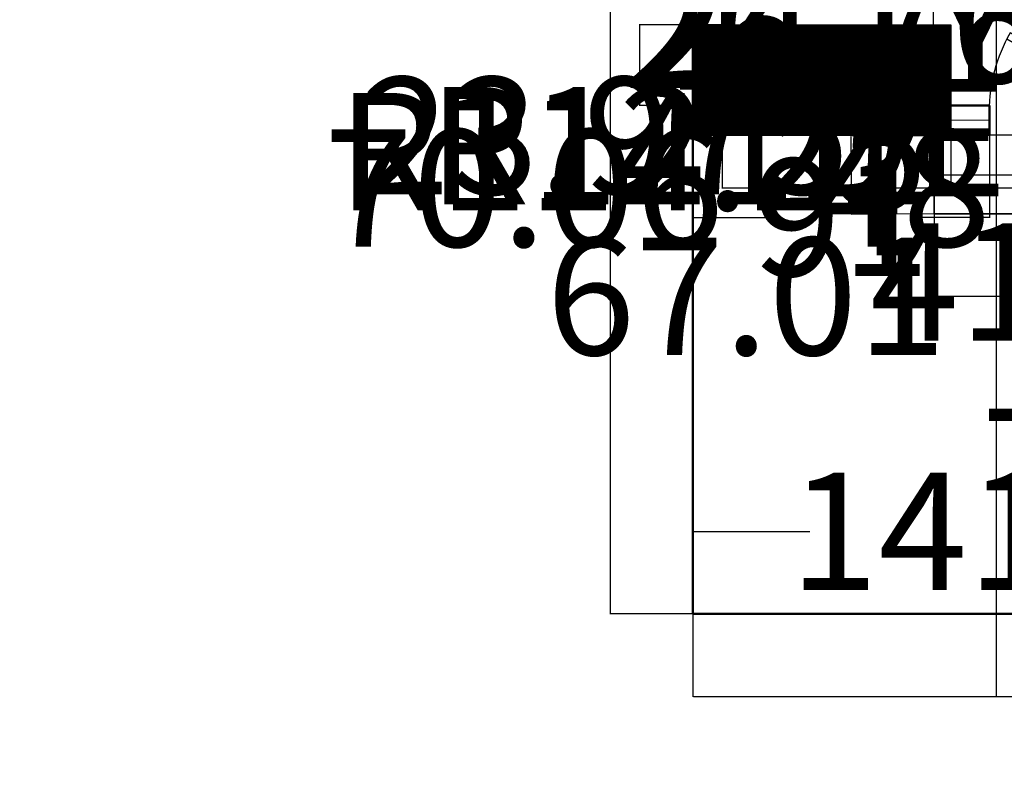
# Model space of a CAD drawing. Units: inches. Extents: x 1173 to 2157, y 515 to 1129.
# Tile 1 of 13: x 1173 to 1475, y 515 to 747. Entities that reach past the tile are written whole.
import ezdxf

# ---------------------------------------------------------------- set-up
doc = ezdxf.new("R2010")
doc.units = ezdxf.units.IN
doc.header["$MEASUREMENT"] = 0
for name, color, linetype, lineweight in [('A-ANNO-DIMS', 2, 'Continuous', 18), ('A-DOOR', 3, 'Continuous', 25), ('A-FLOR', 7, 'Continuous', 25), ('A-FLOR-STRS', 7, 'Continuous', 25), ('A-GLAZ', 4, 'Continuous', 18), ('A-WALL', 7, 'Continuous', 50)]:
    doc.layers.add(name, color=color, linetype=linetype, lineweight=lineweight)
doc.layers.add('A-FLOR-PATT', color=28, linetype='Continuous', lineweight=13, true_color=0x301203)
doc.layers.add('A-WALL-PATT', color=22, linetype='Continuous', lineweight=13, true_color=0xca4b0c)
doc.styles.get("Standard").update_dxf_attribs({"font": 'arial.ttf'})
doc.dimstyles.get("Standard").update_dxf_attribs({"dimtxt": 36, "dimasz": 0.18, "dimexe": 0.18, "dimexo": 0.0625, "dimgap": 0.09, "dimtad": 0, "dimtih": 1, "dimtoh": 1, "dimdec": 0, "dimrnd": 72, "dimzin": 0, "dimdsep": 46, "dimlunit": 3, "dimtxsty": 'Standard', "dimcen": 2, "dimadec": 0, "dimazin": 0, "dimtfac": 1, "dimtdec": 0, "dimtofl": 0, "dimtmove": 0, "dimatfit": 3, "dimfxl": 1, "dimtolj": 1, "dimtzin": 0, "dimarcsym": 0})

# ---------------------------------------------------------------- blocks, each defined once
blk = doc.blocks.new('*U2')
for p, q in [((0, 0), (0, -6)), ((-40, 0), (-40, -6))]:
    blk.add_line(p, q)
blk.add_lwpolyline([(0, 0), (-34.64, 20), (-35.52, 18.48), (-0.88, -1.52)], close=True)
blk.add_arc((0, 0), 40, 150, 180)
blk = doc.blocks.new('WIN-48X9')
blk.add_line((48, 4.5), (0, 4.5))
blk.add_lwpolyline([(0, 9), (48, 9), (48, 0), (0, 0)], close=True)
blk = doc.blocks.new('*D30')
at = {"layer": 'A-ANNO-DIMS', "color": 0, "lineweight": -2, "transparency": 16777216}
for p, q in [((1555.97, 736.03), (1563.78, 736.03)), ((1563.6, 735.85), (1563.6, 729.12)), ((1563.6, 684.97), (1563.6, 691.71)), ((1555.97, 684.79), (1563.78, 684.79))]:
    blk.add_line(p, q, dxfattribs=at)
at = {"layer": 'A-ANNO-DIMS', "color": 0, "transparency": 16777216}
for points in [[(1563.57, 735.85), (1563.63, 735.85), (1563.6, 736.03)], [(1563.57, 684.97), (1563.63, 684.97), (1563.6, 684.79)]]:
    blk.add_solid(points, dxfattribs=at)
at = {"layer": 'Defpoints', "color": 0, "transparency": 16777216}
for p in [(1555.91, 736.03), (1563.6, 736.03), (1555.91, 684.79)]:
    blk.add_point(p, dxfattribs=at)
at = {"layer": 'A-ANNO-DIMS', "color": 0, "transparency": 16777216, "insert": (1563.6, 710.41), "char_height": 36, "attachment_point": 5}
blk.add_mtext('\\A1;DESK 51 TYP.', dxfattribs=at)
blk = doc.blocks.new('*D31')
at = {"layer": 'A-ANNO-DIMS', "color": 0, "lineweight": -2, "transparency": 16777216}
for p, q in [((1529.44, 743.72), (1529.26, 743.72)), ((1529.44, 736.09), (1529.44, 743.9)), ((1555.73, 743.72), (1529.62, 743.72)), ((1555.91, 736.09), (1555.91, 743.9))]:
    blk.add_line(p, q, dxfattribs=at)
at = {"layer": 'A-ANNO-DIMS', "color": 0, "transparency": 16777216}
for points in [[(1529.62, 743.75), (1529.62, 743.69), (1529.44, 743.72)], [(1555.73, 743.75), (1555.73, 743.69), (1555.91, 743.72)]]:
    blk.add_solid(points, dxfattribs=at)
at = {"layer": 'Defpoints', "color": 0, "transparency": 16777216}
for p in [(1529.44, 743.72), (1529.44, 736.03), (1555.91, 736.03)]:
    blk.add_point(p, dxfattribs=at)
at = {"layer": 'A-ANNO-DIMS', "color": 0, "transparency": 16777216, "insert": (1441.24, 743.72), "char_height": 36, "attachment_point": 5}
blk.add_mtext('\\A1;26 TYP.', dxfattribs=at)
blk = doc.blocks.new('*D50')
at = {"layer": 'A-ANNO-DIMS', "color": 0, "lineweight": -2, "transparency": 16777216}
for p, q in [((1603.33, 798.21), (1603.33, 796.59)), ((1613.33, 798.21), (1613.33, 796.59)), ((1603.33, 796.77), (1603.15, 796.77)), ((1613.15, 796.77), (1603.51, 796.77))]:
    blk.add_line(p, q, dxfattribs=at)
at = {"layer": 'A-ANNO-DIMS', "color": 0, "transparency": 16777216}
for points in [[(1603.51, 796.8), (1603.51, 796.74), (1603.33, 796.77)], [(1613.15, 796.8), (1613.15, 796.74), (1613.33, 796.77)]]:
    blk.add_solid(points, dxfattribs=at)
at = {"layer": 'Defpoints', "color": 0, "transparency": 16777216}
for p in [(1603.33, 798.27), (1613.33, 798.27), (1603.33, 796.77)]:
    blk.add_point(p, dxfattribs=at)
at = {"layer": 'A-ANNO-DIMS', "color": 0, "transparency": 16777216, "insert": (1377.9, 796.77), "char_height": 36, "attachment_point": 5}
blk.add_mtext('\\A1;BASIN TAP 10 TYP.', dxfattribs=at)
blk = doc.blocks.new('*D51')
at = {"layer": 'A-ANNO-DIMS', "color": 0, "lineweight": -2, "transparency": 16777216}
for p, q in [((1613.4, 804.77), (1615.01, 804.77)), ((1614.83, 804.59), (1614.83, 798.45)), ((1613.4, 798.27), (1615.01, 798.27)), ((1614.83, 798.09), (1614.65, 798.09)), ((1614.83, 798.27), (1614.83, 798.09))]:
    blk.add_line(p, q, dxfattribs=at)
at = {"layer": 'A-ANNO-DIMS', "color": 0, "transparency": 16777216}
for points in [[(1614.8, 804.59), (1614.86, 804.59), (1614.83, 804.77)], [(1614.8, 798.45), (1614.86, 798.45), (1614.83, 798.27)]]:
    blk.add_solid(points, dxfattribs=at)
at = {"layer": 'Defpoints', "color": 0, "transparency": 16777216}
for p in [(1613.33, 804.77), (1613.33, 798.27), (1614.83, 798.27)]:
    blk.add_point(p, dxfattribs=at)
at = {"layer": 'A-ANNO-DIMS', "color": 0, "transparency": 16777216, "insert": (1541.08, 798.09), "char_height": 36, "attachment_point": 5}
blk.add_mtext('\\A1;7 TYP.', dxfattribs=at)
blk = doc.blocks.new('*D64')
at = {"layer": 'A-ANNO-DIMS', "color": 0, "lineweight": -2, "transparency": 16777216}
for p, q in [((1379.66, 564.22), (1379.66, 538.8)), ((1670.66, 564.22), (1670.66, 538.8)), ((1379.84, 538.98), (1488.47, 538.98)), ((1670.48, 538.98), (1561.86, 538.98))]:
    blk.add_line(p, q, dxfattribs=at)
at = {"layer": 'A-ANNO-DIMS', "color": 0, "transparency": 16777216}
for points in [[(1379.84, 539.01), (1379.84, 538.95), (1379.66, 538.98)], [(1670.48, 539.01), (1670.48, 538.95), (1670.66, 538.98)]]:
    blk.add_solid(points, dxfattribs=at)
at = {"layer": 'Defpoints', "color": 0, "transparency": 16777216}
for p in [(1379.66, 564.28), (1670.66, 564.28), (1670.66, 538.98)]:
    blk.add_point(p, dxfattribs=at)
at = {"layer": 'A-ANNO-DIMS', "color": 0, "transparency": 16777216, "insert": (1525.16, 538.98), "char_height": 36, "attachment_point": 5}
blk.add_mtext('\\A1;291', dxfattribs=at)
blk = doc.blocks.new('*D65')
at = {"layer": 'A-ANNO-DIMS', "color": 0, "lineweight": -2, "transparency": 16777216}
for p, q in [((1379.6, 1053.28), (1354.18, 1053.28)), ((1354.36, 1053.1), (1354.36, 827.25)), ((1354.36, 564.46), (1354.36, 790.31)), ((1379.6, 564.28), (1354.18, 564.28))]:
    blk.add_line(p, q, dxfattribs=at)
at = {"layer": 'A-ANNO-DIMS', "color": 0, "transparency": 16777216}
for points in [[(1354.33, 1053.1), (1354.39, 1053.1), (1354.36, 1053.28)], [(1354.33, 564.46), (1354.39, 564.46), (1354.36, 564.28)]]:
    blk.add_solid(points, dxfattribs=at)
at = {"layer": 'Defpoints', "color": 0, "transparency": 16777216}
for p in [(1354.36, 1053.28), (1379.66, 1053.28), (1379.66, 564.28)]:
    blk.add_point(p, dxfattribs=at)
at = {"layer": 'A-ANNO-DIMS', "color": 0, "transparency": 16777216, "insert": (1354.36, 808.78), "char_height": 36, "attachment_point": 5}
blk.add_mtext('\\A1;489', dxfattribs=at)
blk = doc.blocks.new('*D69')
at = {"layer": 'A-ANNO-DIMS', "color": 0, "lineweight": -2, "transparency": 16777216}
for p, q in [((1472.66, 924.22), (1472.66, 538.8)), ((1520.66, 924.22), (1520.66, 538.8)), ((1472.84, 538.98), (1520.48, 538.98)), ((1520.66, 538.98), (1520.84, 538.98))]:
    blk.add_line(p, q, dxfattribs=at)
at = {"layer": 'A-ANNO-DIMS', "color": 0, "transparency": 16777216}
for points in [[(1472.84, 539.01), (1472.84, 538.95), (1472.66, 538.98)], [(1520.48, 539.01), (1520.48, 538.95), (1520.66, 538.98)]]:
    blk.add_solid(points, dxfattribs=at)
at = {"layer": 'Defpoints', "color": 0, "transparency": 16777216}
for p in [(1472.66, 924.28), (1520.66, 924.28), (1520.66, 538.98)]:
    blk.add_point(p, dxfattribs=at)
at = {"layer": 'A-ANNO-DIMS', "color": 0, "transparency": 16777216, "insert": (1547.48, 538.98), "char_height": 36, "attachment_point": 5}
blk.add_mtext('\\A1;48', dxfattribs=at)
blk = doc.blocks.new('*D70')
at = {"layer": 'A-ANNO-DIMS', "color": 0, "lineweight": -2, "transparency": 16777216}
for p, q in [((1379.66, 711.22), (1379.66, 685.8)), ((1470.66, 711.22), (1470.66, 685.8)), ((1379.84, 685.98), (1402.76, 685.98)), ((1470.48, 685.98), (1447.56, 685.98))]:
    blk.add_line(p, q, dxfattribs=at)
at = {"layer": 'A-ANNO-DIMS', "color": 0, "transparency": 16777216}
for points in [[(1379.84, 686.01), (1379.84, 685.95), (1379.66, 685.98)], [(1470.48, 686.01), (1470.48, 685.95), (1470.66, 685.98)]]:
    blk.add_solid(points, dxfattribs=at)
at = {"layer": 'Defpoints', "color": 0, "transparency": 16777216}
for p in [(1379.66, 711.28), (1470.66, 711.28), (1379.66, 685.98)]:
    blk.add_point(p, dxfattribs=at)
at = {"layer": 'A-ANNO-DIMS', "color": 0, "transparency": 16777216, "insert": (1425.16, 685.98), "char_height": 36, "attachment_point": 5}
blk.add_mtext('\\A1;91', dxfattribs=at)
blk = doc.blocks.new('*D71')
at = {"layer": 'A-ANNO-DIMS', "color": 0, "lineweight": -2, "transparency": 16777216}
for p, q in [((1453.65, 686.97), (1453.65, 661.55)), ((1520.66, 686.97), (1520.66, 661.55)), ((1453.65, 661.73), (1453.47, 661.73)), ((1520.48, 661.73), (1453.83, 661.73))]:
    blk.add_line(p, q, dxfattribs=at)
at = {"layer": 'A-ANNO-DIMS', "color": 0, "transparency": 16777216}
for points in [[(1453.83, 661.76), (1453.83, 661.7), (1453.65, 661.73)], [(1520.48, 661.76), (1520.48, 661.7), (1520.66, 661.73)]]:
    blk.add_solid(points, dxfattribs=at)
at = {"layer": 'Defpoints', "color": 0, "transparency": 16777216}
for p in [(1453.65, 687.03), (1520.66, 687.03), (1453.65, 661.73)]:
    blk.add_point(p, dxfattribs=at)
at = {"layer": 'A-ANNO-DIMS', "color": 0, "transparency": 16777216, "insert": (1396.02, 661.73), "char_height": 36, "attachment_point": 5}
blk.add_mtext('\\A1;67.01', dxfattribs=at)
blk = doc.blocks.new('*D72')
at = {"layer": 'A-ANNO-DIMS', "color": 0, "lineweight": -2, "transparency": 16777216}
for p, q in [((1470.66, 720.22), (1470.66, 694.8)), ((1518.66, 720.22), (1518.66, 694.8)), ((1470.66, 694.98), (1470.48, 694.98)), ((1518.48, 694.98), (1470.84, 694.98))]:
    blk.add_line(p, q, dxfattribs=at)
at = {"layer": 'A-ANNO-DIMS', "color": 0, "transparency": 16777216}
for points in [[(1470.84, 695.01), (1470.84, 694.95), (1470.66, 694.98)], [(1518.48, 695.01), (1518.48, 694.95), (1518.66, 694.98)]]:
    blk.add_solid(points, dxfattribs=at)
at = {"layer": 'Defpoints', "color": 0, "transparency": 16777216}
for p in [(1470.66, 720.28), (1518.66, 720.28), (1470.66, 694.98)]:
    blk.add_point(p, dxfattribs=at)
at = {"layer": 'A-ANNO-DIMS', "color": 0, "transparency": 16777216, "insert": (1443.85, 694.98), "char_height": 36, "attachment_point": 5}
blk.add_mtext('\\A1;48', dxfattribs=at)
blk = doc.blocks.new('*D73')
at = {"layer": 'A-ANNO-DIMS', "color": 0, "lineweight": -2, "transparency": 16777216}
for p, q in [((1379.66, 564.34), (1379.66, 589.76)), ((1379.84, 589.58), (1415.47, 589.58)), ((1520.48, 589.58), (1484.85, 589.58)), ((1520.66, 564.34), (1520.66, 589.76))]:
    blk.add_line(p, q, dxfattribs=at)
at = {"layer": 'A-ANNO-DIMS', "color": 0, "transparency": 16777216}
for points in [[(1379.84, 589.61), (1379.84, 589.55), (1379.66, 589.58)], [(1520.48, 589.61), (1520.48, 589.55), (1520.66, 589.58)]]:
    blk.add_solid(points, dxfattribs=at)
at = {"layer": 'Defpoints', "color": 0, "transparency": 16777216}
for p in [(1520.66, 589.58), (1379.66, 564.28), (1520.66, 564.28)]:
    blk.add_point(p, dxfattribs=at)
at = {"layer": 'A-ANNO-DIMS', "color": 0, "transparency": 16777216, "insert": (1450.16, 589.58), "char_height": 36, "attachment_point": 5}
blk.add_mtext('\\A1;141', dxfattribs=at)
blk = doc.blocks.new('*D77')
at = {"layer": 'A-ANNO-DIMS', "color": 0, "lineweight": -2, "transparency": 16777216}
for p, q in [((1520.6, 645.28), (1495.18, 645.28)), ((1495.36, 645.1), (1495.36, 627.44)), ((1495.36, 573.46), (1495.36, 591.12)), ((1520.6, 573.28), (1495.18, 573.28))]:
    blk.add_line(p, q, dxfattribs=at)
at = {"layer": 'A-ANNO-DIMS', "color": 0, "transparency": 16777216}
for points in [[(1495.33, 645.1), (1495.39, 645.1), (1495.36, 645.28)], [(1495.33, 573.46), (1495.39, 573.46), (1495.36, 573.28)]]:
    blk.add_solid(points, dxfattribs=at)
at = {"layer": 'Defpoints', "color": 0, "transparency": 16777216}
for p in [(1495.36, 645.28), (1520.66, 645.28), (1520.66, 573.28)]:
    blk.add_point(p, dxfattribs=at)
at = {"layer": 'A-ANNO-DIMS', "color": 0, "transparency": 16777216, "insert": (1495.36, 609.28), "char_height": 36, "attachment_point": 5}
blk.add_mtext('\\A1;72', dxfattribs=at)
blk = doc.blocks.new('*D78')
at = {"layer": 'A-ANNO-DIMS', "color": 0, "lineweight": -2, "transparency": 16777216}
for p, q in [((1520.6, 687.03), (1495.18, 687.03)), ((1495.36, 686.85), (1495.36, 684.63)), ((1495.36, 645.46), (1495.36, 647.69)), ((1520.6, 645.28), (1495.18, 645.28))]:
    blk.add_line(p, q, dxfattribs=at)
at = {"layer": 'A-ANNO-DIMS', "color": 0, "transparency": 16777216}
for points in [[(1495.33, 686.85), (1495.39, 686.85), (1495.36, 687.03)], [(1495.33, 645.46), (1495.39, 645.46), (1495.36, 645.28)]]:
    blk.add_solid(points, dxfattribs=at)
at = {"layer": 'Defpoints', "color": 0, "transparency": 16777216}
for p in [(1495.36, 687.03), (1520.66, 687.03), (1520.66, 645.28)]:
    blk.add_point(p, dxfattribs=at)
at = {"layer": 'A-ANNO-DIMS', "color": 0, "transparency": 16777216, "insert": (1495.36, 666.16), "char_height": 36, "attachment_point": 5}
blk.add_mtext('\\A1;41.75', dxfattribs=at)
blk = doc.blocks.new('*D79')
at = {"layer": 'A-ANNO-DIMS', "color": 0, "lineweight": -2, "transparency": 16777216}
for p, q in [((1428.22, 711.05), (1428.04, 711.05)), ((1453.46, 711.01), (1428.04, 710.87)), ((1428.22, 710.87), (1428.22, 711.05)), ((1428.35, 687.08), (1428.22, 710.69)), ((1453.59, 687.03), (1428.17, 686.9))]:
    blk.add_line(p, q, dxfattribs=at)
at = {"layer": 'A-ANNO-DIMS', "color": 0, "transparency": 16777216}
for points in [[(1428.25, 710.69), (1428.19, 710.69), (1428.22, 710.87)], [(1428.38, 687.08), (1428.32, 687.08), (1428.35, 686.9)]]:
    blk.add_solid(points, dxfattribs=at)
at = {"layer": 'Defpoints', "color": 0, "transparency": 16777216}
for p in [(1428.22, 710.87), (1453.52, 711.01), (1453.65, 687.03)]:
    blk.add_point(p, dxfattribs=at)
at = {"layer": 'A-ANNO-DIMS', "color": 0, "transparency": 16777216, "insert": (1352.78, 711.05), "char_height": 36, "attachment_point": 5}
blk.add_mtext('\\A1;23.975', dxfattribs=at)
blk = doc.blocks.new('*D80')
at = {"layer": 'A-ANNO-DIMS', "color": 0, "lineweight": -2, "transparency": 16777216}
for p, q in [((1388.6, 745.04), (1363.18, 745.04)), ((1363.36, 745.04), (1363.36, 745.22)), ((1363.36, 745.22), (1363.54, 745.22)), ((1363.36, 720.46), (1363.36, 744.86)), ((1388.6, 720.28), (1363.18, 720.28))]:
    blk.add_line(p, q, dxfattribs=at)
at = {"layer": 'A-ANNO-DIMS', "color": 0, "transparency": 16777216}
for points in [[(1363.33, 744.86), (1363.39, 744.86), (1363.36, 745.04)], [(1363.33, 720.46), (1363.39, 720.46), (1363.36, 720.28)]]:
    blk.add_solid(points, dxfattribs=at)
at = {"layer": 'Defpoints', "color": 0, "transparency": 16777216}
for p in [(1363.36, 745.04), (1388.66, 745.04), (1388.66, 720.28)]:
    blk.add_point(p, dxfattribs=at)
at = {"layer": 'A-ANNO-DIMS', "color": 0, "transparency": 16777216, "insert": (1424.67, 745.22), "char_height": 36, "attachment_point": 5}
blk.add_mtext('\\A1;24.76', dxfattribs=at)
blk = doc.blocks.new('*D92')
at = {"layer": 'A-ANNO-DIMS', "color": 0, "lineweight": -2, "transparency": 16777216}
for p, q in [((1388.66, 720.22), (1388.66, 694.8)), ((1458.72, 720.22), (1458.72, 694.8)), ((1388.66, 694.98), (1388.48, 694.98)), ((1458.54, 694.98), (1388.84, 694.98))]:
    blk.add_line(p, q, dxfattribs=at)
at = {"layer": 'A-ANNO-DIMS', "color": 0, "transparency": 16777216}
for points in [[(1388.84, 695.01), (1388.84, 694.95), (1388.66, 694.98)], [(1458.54, 695.01), (1458.54, 694.95), (1458.72, 694.98)]]:
    blk.add_solid(points, dxfattribs=at)
at = {"layer": 'Defpoints', "color": 0, "transparency": 16777216}
for p in [(1388.66, 720.28), (1458.72, 720.28), (1388.66, 694.98)]:
    blk.add_point(p, dxfattribs=at)
at = {"layer": 'A-ANNO-DIMS', "color": 0, "transparency": 16777216, "insert": (1327.81, 694.98), "char_height": 36, "attachment_point": 5}
blk.add_mtext('\\A1;70.06', dxfattribs=at)
blk = doc.blocks.new('*D103')
at = {"layer": 'A-ANNO-DIMS', "color": 0, "lineweight": -2, "transparency": 16777216}
for p, q in [((1453.43, 899.94), (1453.43, 903.94)), ((1451.43, 901.94), (1455.43, 901.94)), ((1453.43, 708.02), (1453.43, 780.56)), ((1453.25, 708.02), (1453.43, 708.02))]:
    blk.add_line(p, q, dxfattribs=at)
at = {"layer": 'A-ANNO-DIMS', "color": 0, "transparency": 16777216}
blk.add_solid([(1453.4, 780.56), (1453.46, 780.56), (1453.43, 780.74)], dxfattribs=at)
at = {"layer": 'Defpoints', "color": 0, "transparency": 16777216}
for p in [(1453.43, 901.94), (1453.43, 780.74)]:
    blk.add_point(p, dxfattribs=at)
at = {"layer": 'A-ANNO-DIMS', "color": 0, "transparency": 16777216, "insert": (1375.38, 708.02), "char_height": 36, "attachment_point": 5}
blk.add_mtext('\\A1;R121.2', dxfattribs=at)
blk = doc.blocks.new('*D104')
at = {"layer": 'A-ANNO-DIMS', "color": 0, "lineweight": -2, "transparency": 16777216}
for p, q in [((1453.43, 886.99), (1453.43, 890.99)), ((1451.43, 888.99), (1455.43, 888.99)), ((1453.43, 706.19), (1453.43, 774.56)), ((1453.25, 706.19), (1453.43, 706.19))]:
    blk.add_line(p, q, dxfattribs=at)
at = {"layer": 'A-ANNO-DIMS', "color": 0, "transparency": 16777216}
blk.add_solid([(1453.4, 774.56), (1453.46, 774.56), (1453.43, 774.74)], dxfattribs=at)
at = {"layer": 'Defpoints', "color": 0, "transparency": 16777216}
for p in [(1453.43, 888.99), (1453.43, 774.74)]:
    blk.add_point(p, dxfattribs=at)
at = {"layer": 'A-ANNO-DIMS', "color": 0, "transparency": 16777216, "insert": (1361.08, 706.19), "char_height": 36, "attachment_point": 5}
blk.add_mtext('\\A1;R114.25', dxfattribs=at)

msp = doc.modelspace()

# ---------------------------------------------------------------- hatches: boundary and pattern name
at = {"layer": 'A-FLOR-PATT'}
h = msp.add_hatch(dxfattribs=at)
h.set_pattern_fill('ANSI31', color=256)
h.paths.add_polyline_path([(1458.7214, 745.0427), (1388.6635, 745.0427), (1388.6635, 720.2805), (1458.7214, 720.2805)])
at = {"layer": 'A-WALL-PATT'}
h = msp.add_hatch(dxfattribs=at)
h.set_pattern_fill('ANSI31', color=256)
h.paths.add_polyline_path([(1388.6635, 933.2805), (1388.6635, 1044.2805), (1413.7618, 1044.2805), (1413.7618, 1053.2805), (1379.6635, 1053.2805), (1379.6635, 894.1606), (1388.6635, 894.1606), (1388.6635, 924.2805), (1472.6635, 924.2805), (1472.6635, 933.2805)])
h.paths.add_polyline_path([(1520.6635, 1044.2805), (1520.6635, 1014.7866), (1520.6635, 1005.1794), (1520.7714, 1005.1794), (1520.7714, 956.4707), (1520.6635, 924.2805), (1529.6635, 924.2805), (1529.6635, 931.4788), (1529.6635, 1044.2805), (1530.8474, 1044.2805), (1570.9543, 1044.2805), (1570.9543, 1053.2805), (1461.7618, 1053.2805), (1461.7618, 1044.2805)])
h.paths.add_polyline_path([(1618.9543, 1053.2805), (1618.9543, 1044.2805), (1661.6635, 1044.2805), (1661.6635, 1043.7367), (1661.6635, 1032.8874), (1670.6635, 1032.8874), (1670.6635, 1053.2805)])
h.paths.add_polyline_path([(1661.6635, 933.2805), (1661.6635, 927.8377), (1661.6635, 924.2805), (1661.6635, 918.9156), (1670.6635, 918.9156), (1670.6635, 984.8874), (1661.6635, 984.8874), (1661.6635, 978.3712)])
h.paths.add_polyline_path([(1670.6635, 894.9156), (1661.6635, 894.9156), (1661.6635, 890.0349), (1661.9328, 890.0349), (1661.9328, 870.079), (1661.6635, 864.2805), (1589.6635, 864.2805), (1589.6635, 924.2805), (1625.553, 924.2805, -0.02455299), (1625.3782, 927.8377), (1625.3782, 933.2805), (1577.6635, 933.2805), (1577.6635, 924.2805), (1580.6635, 924.2805), (1580.6635, 855.2805), (1586.1062, 855.2805), (1589.6635, 855.2805), (1661.6635, 855.2805), (1661.6635, 826.5597), (1670.6635, 826.5597)])
h.paths.add_polyline_path([(1670.6635, 802.5597), (1661.6635, 802.5597), (1661.6635, 795.2805), (1589.6635, 795.2805), (1589.6635, 819.17, -0.02455299), (1586.1062, 818.9952), (1580.6635, 818.9952), (1580.6635, 795.2805), (1577.6635, 795.2805), (1577.6635, 786.2805), (1661.6635, 786.2805), (1661.6635, 778.5597), (1661.6635, 742.6973), (1670.6635, 742.6973)])
h.paths.add_polyline_path([(1661.6635, 654.2805), (1625.1498, 654.2805), (1625.1498, 645.2805), (1661.3656, 645.2805), (1661.6635, 645.2805), (1661.6635, 573.2805), (1520.6635, 573.2805), (1520.6635, 564.2805), (1670.6635, 564.2805), (1670.6635, 694.6973), (1661.6635, 694.6973)])
h.paths.add_polyline_path([(1529.4367, 733.4702, -0.06854064), (1529.6635, 734.2623), (1529.6635, 795.2805), (1520.6635, 795.2805), (1520.6635, 645.2805), (1577.1498, 645.2805), (1577.1498, 654.2805), (1529.6635, 654.2805), (1529.6635, 686.5626, -0.06854064), (1529.4367, 687.3547)])
h.paths.add_polyline_path([(1379.6635, 711.2805), (1388.6635, 711.2805), (1458.7214, 711.2805), (1458.7214, 720.2805), (1410.7214, 720.2805), (1388.6635, 720.2805), (1388.6635, 745.0427), (1379.6635, 745.0427)])
h.paths.add_polyline_path([(1388.6635, 846.1606), (1379.6635, 846.1606), (1379.6635, 793.0427), (1388.6635, 793.0427)])

# ---------------------------------------------------------------- linework, layer by layer
at = {"layer": 'A-FLOR'}
for p, q in [((1379.6635, 711.2805), (1453.5214, 711.0087)), ((1379.6635, 564.2805), (1379.6635, 711.2805)), ((1379.6635, 711.2805), (1386.9581, 711.2537)), ((1384.1635, 711.2805), (1379.6635, 711.2805)), ((1453.5214, 711.0087), (1453.6517, 687.0336)), ((1453.6517, 687.0336), (1520.6635, 687.0336)), ((1520.6635, 564.2805), (1379.6635, 564.2805))]:
    msp.add_line(p, q, dxfattribs=at)
msp.add_lwpolyline([(1388.6635, 745.0427), (1458.7214, 745.0427), (1458.7214, 720.2805), (1388.6635, 720.2805)], close=True, dxfattribs=at)
at = {"layer": 'A-FLOR-STRS'}
for p, q in [((1453.5214, 711.0087), (1453.5214, 698.7437)), ((1470.6635, 711.2805), (1520.6635, 711.2805)), ((1453.6517, 699.0155), (1520.6635, 699.0155)), ((1453.6517, 687.0336), (1453.6517, 699.0155)), ((1520.6635, 687.0336), (1453.6517, 687.0336))]:
    msp.add_line(p, q, dxfattribs=at)
at = {"layer": 'A-GLAZ'}
msp.add_line((1458.7214, 715.7805), (1470.5017, 715.7805), dxfattribs=at)
msp.add_lwpolyline([(1410.7214, 720.2805), (1458.7214, 720.2805), (1458.7214, 711.2805), (1410.7214, 711.2805)], dxfattribs=at)
at = {"layer": 'A-WALL'}
for p, q in [((1388.6635, 924.2805), (1388.6635, 720.2805)), ((1470.6635, 720.2805), (1388.6635, 720.2805)), ((1470.6635, 711.2805), (1470.6635, 720.2805)), ((1388.6635, 711.2805), (1379.6635, 711.2805)), ((1470.6635, 711.2805), (1388.6635, 711.2805))]:
    msp.add_line(p, q, dxfattribs=at)
msp.add_lwpolyline([(1379.6635, 564.2805), (1670.6635, 564.2805), (1670.6635, 1053.2805), (1379.6635, 1053.2805)], close=True, dxfattribs=at)

# ---------------------------------------------------------------- block references
at = {"layer": 'A-DOOR', "xscale": 1.204044770816111, "yscale": 1.204044770816111, "zscale": 1.204044770816111}
msp.add_blockref('*U2', (1518.6635, 718.5048), dxfattribs=at)
at = {"layer": 'A-GLAZ', "rotation": 269.9999999999995}
msp.add_blockref('WIN-48X9', (1379.6635, 793.0427), dxfattribs=at)

# ---------------------------------------------------------------- dimensions: what is measured, and where the dimension line sits
at = {"layer": 'A-ANNO-DIMS'}
for base, p1, p2, angle, override, picture, middle in [((1354.361, 1053.2805), (1379.6635, 564.2805), (1379.6635, 1053.2805), 90, {"dimdec": 0, "dimlfac": 1, "dimrnd": 0, "dimzin": 0, "dimdsep": 46, "dimlunit": 2}, '*D65', (1354.361, 808.7805)), ((1363.361, 745.0427), (1388.6635, 720.2805), (1388.6635, 745.0427), 90, {"dimdec": 2, "dimlfac": 1, "dimrnd": 0, "dimzin": 0, "dimdsep": 46, "dimlunit": 2}, '*D80', (1424.6664, 745.2227)), ((1428.2193, 710.8711), (1453.6517, 687.0336), (1453.5214, 711.0087), 90.311494, {"dimdec": 3, "dimlfac": 1, "dimrnd": 0, "dimzin": 0, "dimdsep": 46, "dimlunit": 2}, '*D79', (1352.7805, 711.0511)), ((1388.6635, 694.978), (1458.7214, 720.2805), (1388.6635, 720.2805), 180, {"dimdec": 2, "dimlfac": 1, "dimrnd": 0, "dimzin": 0, "dimdsep": 46, "dimlunit": 2}, '*D92', (1327.8123, 694.978)), ((1470.6635, 694.978), (1518.6635, 720.2805), (1470.6635, 720.2805), 180, {"dimdec": 0, "dimlfac": 1, "dimrnd": 0, "dimzin": 0, "dimdsep": 46, "dimlunit": 2}, '*D72', (1443.8478, 694.978)), ((1379.6635, 685.978), (1470.6635, 711.2805), (1379.6635, 711.2805), 180, {"dimdec": 0, "dimlfac": 1, "dimrnd": 0, "dimzin": 0, "dimdsep": 46, "dimlunit": 2}, '*D70', (1425.1635, 685.978)), ((1495.361, 687.0336), (1520.6635, 645.2805), (1520.6635, 687.0336), 90, {"dimdec": 2, "dimlfac": 1, "dimrnd": 0, "dimzin": 0, "dimdsep": 46, "dimlunit": 2}, '*D78', (1495.361, 666.1571)), ((1453.6517, 661.7311), (1520.6635, 687.0336), (1453.6517, 687.0336), 180, {"dimdec": 2, "dimlfac": 1, "dimrnd": 0, "dimzin": 0, "dimdsep": 46, "dimlunit": 2}, '*D71', (1396.0175, 661.7311)), ((1495.361, 645.2805), (1520.6635, 573.2805), (1520.6635, 645.2805), 90, {"dimdec": 0, "dimlfac": 1, "dimrnd": 0, "dimzin": 0, "dimdsep": 46, "dimlunit": 2}, '*D77', (1495.361, 609.2805))]:
    dim = msp.add_linear_dim(base=base, p1=p1, p2=p2, angle=angle, dimstyle='Standard', override=override, dxfattribs=at)
    dim.commit()
    dim.dimension.update_dxf_attribs({"geometry": picture, "text_midpoint": middle})
for base, p1, p2, picture, middle in [((1520.6635, 538.978), (1472.6635, 924.2805), (1520.6635, 924.2805), '*D69', (1547.4792, 538.978)), ((1520.6635, 589.583), (1379.6635, 564.2805), (1520.6635, 564.2805), '*D73', (1450.1635, 589.583)), ((1670.6635, 538.978), (1379.6635, 564.2805), (1670.6635, 564.2805), '*D64', (1525.1635, 538.978))]:
    dim = msp.add_linear_dim(base=base, p1=p1, p2=p2, dimstyle='Standard', override={"dimdec": 0, "dimlfac": 1, "dimrnd": 0, "dimzin": 0, "dimdsep": 46, "dimlunit": 2}, dxfattribs=at)
    dim.commit()
    dim.dimension.update_dxf_attribs({"geometry": picture, "text_midpoint": middle})
for base, p1, p2, angle, text, picture, middle in [((1603.3335, 796.7679), (1613.3335, 798.2679), (1603.3335, 798.2679), 180, 'BASIN TAP <> TYP.', '*D50', (1377.9039, 796.7679)), ((1614.8335, 798.2679), (1613.3335, 804.768), (1613.3335, 798.2679), 270, '<> TYP.', '*D51', (1541.0778, 798.0879)), ((1529.4367, 743.7181), (1555.9105, 736.0322), (1529.4367, 736.0322), 180, '<> TYP.', '*D31', (1441.2418, 743.7181)), ((1563.5964, 736.0322), (1555.9105, 684.7928), (1555.9105, 736.0322), 90, 'DESK <> TYP.', '*D30', (1563.5964, 710.4125))]:
    dim = msp.add_linear_dim(base=base, p1=p1, p2=p2, angle=angle, text=text, dimstyle='Standard', override={"dimdec": 0, "dimlfac": 1, "dimrnd": 0, "dimzin": 0, "dimdsep": 46, "dimlunit": 2}, dxfattribs=at)
    dim.commit()
    dim.dimension.update_dxf_attribs({"geometry": picture, "text_midpoint": middle})
for center, mpoint, override, picture, middle in [((1453.4344, 901.9366), (1453.434, 780.7398), {"dimdec": 1, "dimlfac": 1, "dimrnd": 0, "dimzin": 0, "dimdsep": 46, "dimlunit": 2}, '*D103', (1375.3807, 708.0217)), ((1453.4344, 888.9898), (1453.434, 774.7398), {"dimdec": 2, "dimlfac": 1, "dimrnd": 0, "dimzin": 0, "dimdsep": 46, "dimlunit": 2}, '*D104', (1361.0764, 706.1898))]:
    dim = msp.add_radius_dim(center=center, mpoint=mpoint, dimstyle='Standard', override=override, dxfattribs=at)
    dim.commit()
    dim.dimension.update_dxf_attribs({"geometry": picture, "text_midpoint": middle, "dimtype": 164})

doc.saveas('drawing.dxf')
